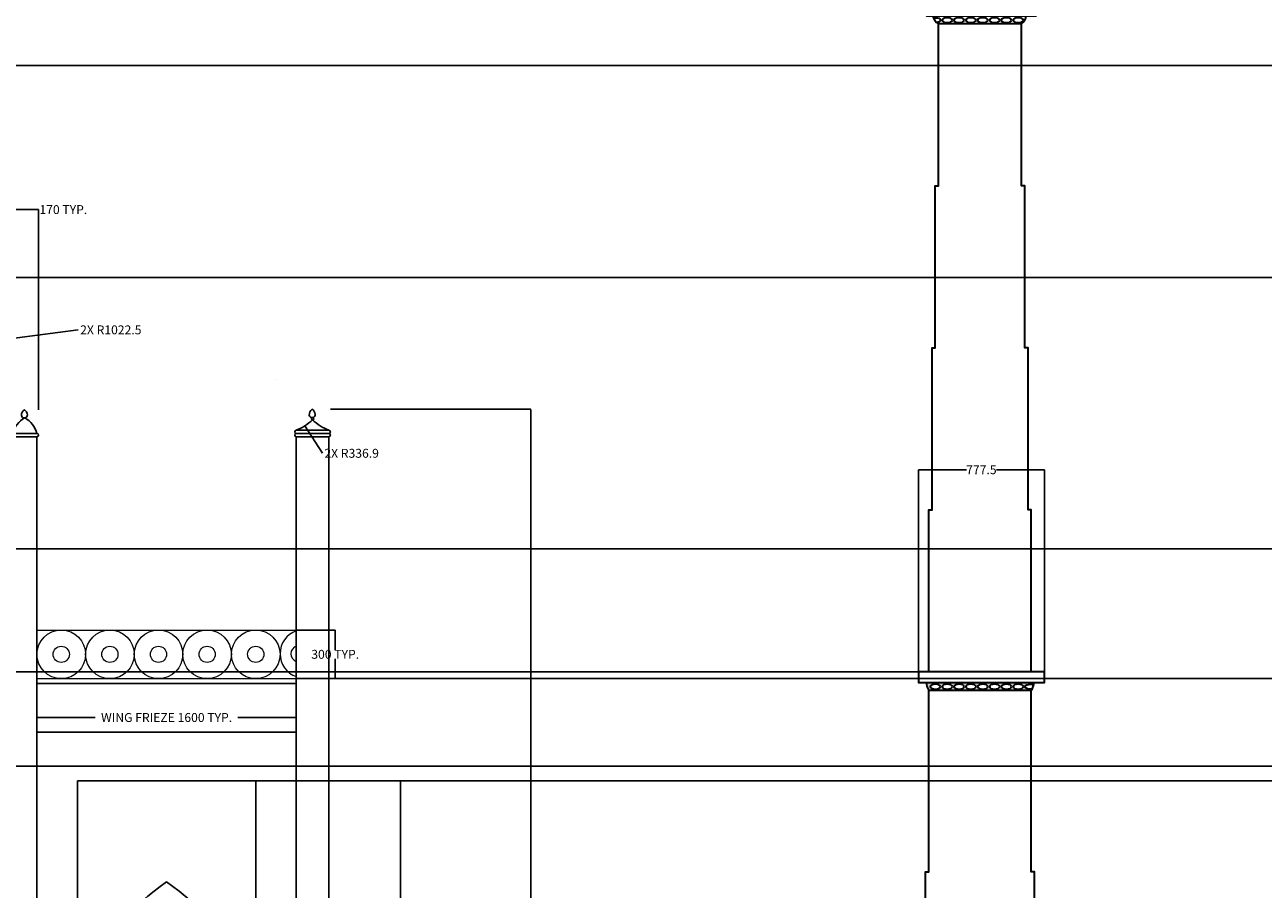
# Model space of a CAD drawing. Units: millimetres. Extents: x 8570 to 49085, y 3782 to 24863.
# Tile 9 of 15: x 27529 to 35169, y 12499 to 17835. Entities that reach past the tile are written whole.
import ezdxf

# ---------------------------------------------------------------- set-up
doc = ezdxf.new("R2010")
doc.units = ezdxf.units.MM
doc.header["$MEASUREMENT"] = 0
doc.header["$PDMODE"] = 3
for name, color, linetype, lineweight in [('A-ANNO-DIMS', 2, 'Continuous', 18), ('A-ELEV', 7, 'Continuous', 25), ('A-ELEV-ARCH', 7, 'Continuous', 25), ('A-ELEV-MNRT', 7, 'Continuous', 30), ('A-ELEV-ORNM', 7, 'Continuous', 13), ('A-ELEV-PIER', 7, 'Continuous', 25)]:
    doc.layers.add(name, color=color, linetype=linetype, lineweight=lineweight)
doc.styles.get("Standard").update_dxf_attribs({"font": 'arial.ttf'})
doc.dimstyles.get("Standard").update_dxf_attribs({"dimtxt": 55, "dimasz": 0.18, "dimexe": 0.18, "dimexo": 0.0625, "dimgap": 0.09, "dimtad": 0, "dimtih": 1, "dimtoh": 1, "dimdec": 0, "dimzin": 0, "dimdsep": 46, "dimtxsty": 'Standard', "dimcen": 0.09, "dimadec": 0, "dimazin": 0, "dimtfac": 1, "dimtdec": 0, "dimtofl": 0, "dimtmove": 0, "dimatfit": 3, "dimfxl": 1, "dimtolj": 1, "dimtzin": 0, "dimarcsym": 0})

# ---------------------------------------------------------------- blocks, each defined once
blk = doc.blocks.new('MINARET-ELEV')
h = blk.add_hatch(color=256)
h.dxf.hatch_style = 1
edge = h.paths.add_edge_path()
edge.add_arc((788.1, 7879), 96, 347.52389, 357.31225, ccw=False)
edge.add_ellipse((859.2, 7847.7), major_axis=(31.8, 0), ratio=0.472441, start_angle=385.01443, end_angle=315.51296)
edge.add_arc((788.1, 7879), 96, 325.26025, 332.17741, ccw=False)
edge.add_line((867, 7824.3), (235, 7824.3))
edge.add_arc((313.9, 7879), 96, 182.68775, 214.73975, ccw=False)
edge.add_line((218, 7874.5), (884, 7874.5))
edge = h.paths.add_edge_path(flags=16)
edge.add_ellipse((494.2, 7847.7), major_axis=(31.8, 0), ratio=0.472441, start_angle=0, end_angle=360, ccw=False)
edge = h.paths.add_edge_path(flags=16)
edge.add_ellipse((567.2, 7847.7), major_axis=(31.8, 0), ratio=0.472441, start_angle=0, end_angle=360, ccw=False)
edge = h.paths.add_edge_path(flags=16)
edge.add_ellipse((421.2, 7847.7), major_axis=(31.8, 0), ratio=0.472441, start_angle=0, end_angle=360, ccw=False)
edge = h.paths.add_edge_path(flags=16)
edge.add_ellipse((640.2, 7847.7), major_axis=(31.8, 0), ratio=0.472441, start_angle=0, end_angle=360, ccw=False)
edge = h.paths.add_edge_path(flags=16)
edge.add_ellipse((348.2, 7847.7), major_axis=(31.8, 0), ratio=0.472441, start_angle=0, end_angle=360, ccw=False)
edge = h.paths.add_edge_path(flags=16)
edge.add_ellipse((713.2, 7847.7), major_axis=(31.8, 0), ratio=0.472441, start_angle=0, end_angle=360, ccw=False)
edge = h.paths.add_edge_path(flags=16)
edge.add_ellipse((275.2, 7847.7), major_axis=(31.8, 0), ratio=0.472441, start_angle=0, end_angle=360, ccw=False)
edge = h.paths.add_edge_path(flags=16)
edge.add_ellipse((786.2, 7847.7), major_axis=(31.8, 0), ratio=0.472441, start_angle=0, end_angle=360, ccw=False)
h = blk.add_hatch(color=256)
h.dxf.hatch_style = 1
edge = h.paths.add_edge_path()
edge.add_arc((940, 4615.3), 25, 270, 450, ccw=False)
edge.add_line((940, 4590.3), (160, 4590.3))
edge.add_arc((160, 4615.3), 25, 217.6761, 270, ccw=False)
edge.add_ellipse((127.2, 4613.7), major_axis=(31.8, 0), ratio=0.472441, start_angle=313.43175, end_angle=411.74889)
edge.add_arc((160, 4615.3), 25, 450, 510.08055, ccw=False)
edge.add_line((160, 4640.3), (940, 4640.3))
edge = h.paths.add_edge_path(flags=16)
edge.add_ellipse((347.2, 4613.7), major_axis=(31.8, 0), ratio=0.472441, start_angle=0, end_angle=360, ccw=False)
edge = h.paths.add_edge_path(flags=16)
edge.add_ellipse((420.2, 4613.7), major_axis=(31.8, 0), ratio=0.472441, start_angle=0, end_angle=360, ccw=False)
edge = h.paths.add_edge_path(flags=16)
edge.add_ellipse((274.2, 4613.7), major_axis=(31.8, 0), ratio=0.472441, start_angle=0, end_angle=360, ccw=False)
edge = h.paths.add_edge_path(flags=16)
edge.add_ellipse((493.2, 4613.7), major_axis=(31.8, 0), ratio=0.472441, start_angle=0, end_angle=360, ccw=False)
edge = h.paths.add_edge_path(flags=16)
edge.add_ellipse((198.8, 4613.7), major_axis=(31.8, 0), ratio=0.472441, start_angle=0, end_angle=360, ccw=False)
edge = h.paths.add_edge_path(flags=16)
edge.add_ellipse((566.2, 4613.7), major_axis=(31.8, 0), ratio=0.472441, start_angle=0, end_angle=360, ccw=False)
edge = h.paths.add_edge_path(flags=16)
edge.add_ellipse((639.2, 4613.7), major_axis=(31.8, 0), ratio=0.472441, start_angle=0, end_angle=360, ccw=False)
edge = h.paths.add_edge_path(flags=16)
edge.add_ellipse((712.2, 4613.7), major_axis=(31.8, 0), ratio=0.472441, start_angle=0, end_angle=360, ccw=False)
edge = h.paths.add_edge_path(flags=16)
edge.add_ellipse((785.2, 4613.7), major_axis=(31.8, 0), ratio=0.472441, start_angle=0, end_angle=360, ccw=False)
edge = h.paths.add_edge_path(flags=16)
edge.add_ellipse((858.2, 4613.7), major_axis=(31.8, 0), ratio=0.472441, start_angle=0, end_angle=360, ccw=False)
edge = h.paths.add_edge_path(flags=16)
edge.add_ellipse((931.2, 4613.7), major_axis=(31.8, 0), ratio=0.472441, start_angle=0, end_angle=360, ccw=False)
for p, q in [((851, 12922), (257.5, 12922)), ((257.5, 12922), (257.5, 12872)), ((851, 12922), (851, 12872)), ((851, 12897), (257.5, 12897)), ((851, 12872), (257.5, 12872)), ((298, 12162), (298, 12872)), ((556.7, 12843), (552, 12843)), ((815.5, 12162), (815.5, 12872)), ((348, 12162), (348, 12766.4)), ((423, 12162), (423, 12760.1)), ((765.5, 12162), (765.5, 12770.9)), ((690.5, 12162), (690.5, 12757.3)), ((815.5, 12162), (298, 12162)), ((807, 11939), (295, 11939)), ((867, 7824.3), (235, 7824.3)), ((867, 7824.3), (235, 7824.3)), ((160, 4590.3), (940, 4590.3)), ((165, 4590.3), (935, 4590.3)), ((905, 4590.3), (195, 4590.3)), ((300, 0), (300, 1321)), ((800, 0), (800, 1321)), ((1100, 0), (1100, 1321))]:
    blk.add_line(p, q)
blk.add_lwpolyline([(512, 13519.5, -0.216309), (551.3, 13585.8, -0.244698), (591, 13509.3, -0.244698)], format="xyb")
for points in [[(554, 13300, -0.140093), (458.9, 13405.9, -0.184272)], [(554, 13300, 0.140093), (646.7, 13408, 0.184272)]]:
    blk.add_lwpolyline(points, format="xyb", close=True)
for points in [[(815.5, 12072.5), (298, 12072.5), (298, 12162), (815.5, 12162)], [(898, 12072.5), (220.5, 12072.5), (220.5, 11989.2), (898, 11989.2)], [(948, 7939), (170.5, 7939), (170.5, 7874.5), (948, 7874.5)], [(997, 4705), (119.5, 4705), (119.5, 4640.5), (997, 4640.5)]]:
    blk.add_lwpolyline(points, close=True)
for points in [[(235, 7939), (235, 8939), (255, 8939), (255, 9939), (275, 9939), (275, 10939), (295, 10939), (295, 11939)], [(867, 7939), (867, 8939), (847, 8939), (847, 9939), (827, 9939), (827, 10939), (807, 10939), (807, 11939)], [(195, 4705), (195, 5705), (215, 5705), (215, 6705), (235, 6705), (235, 7824.3)], [(907, 4705), (907, 5705), (887, 5705), (887, 6705), (867, 6705), (867, 7824.3)], [(135, 1321), (135, 2321), (155, 2321), (155, 3321), (175, 3321), (175, 4321), (195, 4321), (195, 4590.3)], [(965, 1321), (965, 2321), (945, 2321), (945, 3321), (925, 3321), (925, 4321), (905, 4321), (905, 4590.3)], [(0, 1321), (1100, 1321)], [(0, 1246), (1100, 1246)]]:
    blk.add_lwpolyline(points)
for centre, radius in [((552, 13415.4), 63.1), ((554, 13261.5), 38.5)]:
    blk.add_circle(centre, radius)
for centre, radius, start, end in [((552, 13518.5), 40.1, 178.61203, 346.69346), ((554, 12961.3), 261.7, 351.36698, 188.63302), ((330.8, 12000.6), 71.3, 189.21146, 239.80255), ((759.2, 12000.8), 78.1, 307.68318, 351.42034), ((313.9, 7879), 96, 182.68775, 214.73975), ((788.1, 7879), 96, 325.26025, 357.31225), ((160, 4615.3), 25, 90, 270), ((940, 4615.3), 25, 270, 90)]:
    blk.add_arc(centre, radius, start, end)
at = {"extrusion": (0, 0, -1)}
for centre, start_param, end_param in [((275.2, 11962.4), -1.939365, 1.327018), ((348.2, 11962.4), -6.283185, 0), ((421.2, 11962.4), -6.283185, 0), ((494.2, 11962.4), -6.283185, 0), ((567.2, 11962.4), -6.283185, 0), ((640.2, 11962.4), -6.283185, 0), ((713.2, 11962.4), -6.283185, 0), ((786.2, 11962.4), -6.283185, 0), ((275.2, 7847.7), -6.283185, 0), ((348.2, 7847.7), -6.283185, 0), ((421.2, 7847.7), -6.283185, 0), ((494.2, 7847.7), -6.283185, 0), ((567.2, 7847.7), -6.283185, 0), ((640.2, 7847.7), -6.283185, 0), ((713.2, 7847.7), -6.283185, 0), ((786.2, 7847.7), -6.283185, 0), ((859.2, 7847.7), -5.160703, -0.779193), ((127.2, 4613.7), -1.214257, 1.150222), ((198.8, 4613.7), -6.283185, 0), ((274.2, 4613.7), -6.283185, 0), ((347.2, 4613.7), -6.283185, 0), ((420.2, 4613.7), -6.283185, 0), ((493.2, 4613.7), -6.283185, 0), ((566.2, 4613.7), -6.283185, 0), ((639.2, 4613.7), -6.283185, 0), ((712.2, 4613.7), -6.283185, 0), ((785.2, 4613.7), -6.283185, 0), ((858.2, 4613.7), -6.283185, 0), ((931.2, 4613.7), -6.283185, 0)]:
    blk.add_ellipse(centre, major_axis=(31.8, 0), ratio=0.472441, start_param=start_param, end_param=end_param, dxfattribs=at)
for points in [[(554.4, 12843), (553.6, 12843), (500.8, 12843), (391.9, 12680.1), (321.9, 12795.7), (298, 12872)], [(554.4, 12843), (555.2, 12843), (607.9, 12843), (716.8, 12680.1), (786.9, 12795.7), (815.5, 12872)]]:
    blk.add_open_spline(points, degree=3, knots=[136.061972, 136.061972, 136.061972, 136.061972, 139.000899, 330.944902, 463.724089, 463.724089, 463.724089, 463.724089])
blk = doc.blocks.new('PAVILION-EDGE-PINNACLE')
for p, q in [((10, 8089.5), (160, 8089.5)), ((10, 0), (10, 8069.5)), ((10, 8069.5), (160, 8069.5)), ((160, 0), (160, 8069.5)), ((160, 0), (160, 6876.5)), ((10, 0), (10, 6246.5))]:
    blk.add_line(p, q)
blk.add_lwpolyline([(101.6, 8204.8, 0.216309), (82.9, 8236.3, 0.244698), (64, 8200, 0.244698)], format="xyb")
for centre, radius, start, end in [((153, 8055.1), 147, 117.52778, 166.47476), ((82.6, 8204.4), 19, 193.30654, 1.38797), ((17, 8055.1), 147, 13.52524, 62.47222), ((10, 8079.5), 10, 90, 270), ((160, 8079.5), 10, 270, 90)]:
    blk.add_arc(centre, radius, start, end)
blk = doc.blocks.new('WING-END-PINNACLE')
for p, q in [((10, 8109.5), (210, 8109.5)), ((10, 8089.5), (210, 8089.5)), ((10, 0), (10, 8069.5)), ((10, 8069.5), (210, 8069.5)), ((210, 0), (210, 8069.5))]:
    blk.add_line(p, q)
blk.add_lwpolyline([(127.1, 8207.4, 0.216309), (108.4, 8238.9, 0.244698), (89.5, 8202.5, 0.244698)], format="xyb")
blk.add_circle((110.5, 8181), 7.02)
for centre, radius, start, end in [((108.1, 8206.9), 19, 193.30654, 1.38797), ((10, 8099.5), 10, 90, 270), ((-119.7, 8420.4), 336.9, 292.6494, 312.99463), ((340.2, 8421.1), 337.7, 227.0303, 247.32566), ((210, 8099.5), 10, 270, 90), ((10, 8079.5), 10, 90, 270), ((210, 8079.5), 10, 270, 90)]:
    blk.add_arc(centre, radius, start, end)
blk = doc.blocks.new('WING-RING-FRIEZE')
for p, q in [((0, 300), (1600, 300)), ((0, 0), (1600, 0))]:
    blk.add_line(p, q)
for centre, radius in [((150, 150), 150), ((450, 150), 150), ((750, 150), 150), ((1050, 150), 150), ((1349.9, 150), 150), ((150, 150), 50), ((450, 150), 50), ((750, 150), 50), ((1050, 150), 50), ((1349.9, 150), 50)]:
    blk.add_circle(centre, radius)
for centre, radius in [((1649.9, 153.7), 150), ((1616.6, 153.7), 50)]:
    blk.add_arc(centre, radius, 109.41717, 250.58283)
blk = doc.blocks.new('WING-TALL-ARCH')
for p, q in [((0, 5946.5), (1100, 5946.5)), ((0, 0), (0, 5946.5)), ((1100, 0), (1100, 5946.5)), ((0, 3123.2), (1100, 3123.2))]:
    blk.add_line(p, q)
for points in [[(47.9, 4748, -0.124525), (550, 5321.3, -0.124525)], [(1052.1, 4748, 0.124525), (550, 5321.3, 0.124525)]]:
    blk.add_lwpolyline(points, format="xyb")
for centre, start, end in [((817.4, 4459.8), 159.46554, 174.14569), ((282.6, 4459.8), 5.85431, 20.53446)]:
    blk.add_arc(centre, 821.7, start, end)
blk = doc.blocks.new('*D15')
at = {"layer": 'A-ANNO-DIMS', "color": 0, "lineweight": -2, "transparency": 16777216}
for p, q in [((33971.1, 19487.3), (36009.1, 19487.3)), ((36008.9, 19487.1), (36008.9, 12722.6)), ((36008.9, 5901.7), (36008.9, 12666.2)), ((33971.1, 5901.5), (36009.1, 5901.5))]:
    blk.add_line(p, q, dxfattribs=at)
at = {"layer": 'A-ANNO-DIMS', "color": 0, "transparency": 16777216}
for points in [[(36008.8, 19487.1), (36008.9, 19487.1), (36008.9, 19487.3)], [(36008.8, 5901.7), (36008.9, 5901.7), (36008.9, 5901.5)]]:
    blk.add_solid(points, dxfattribs=at)
at = {"layer": 'Defpoints', "color": 0, "transparency": 16777216}
for p in [(33971, 19487.3), (36008.9, 19487.3), (33971, 5901.5)]:
    blk.add_point(p, dxfattribs=at)
at = {"layer": 'A-ANNO-DIMS', "color": 0, "transparency": 16777216, "insert": (36008.9, 12694.4), "char_height": 55, "attachment_point": 5}
blk.add_mtext('\\A1;MINARET 13586 TYP.', dxfattribs=at)
blk = doc.blocks.new('*D22')
at = {"layer": 'A-ANNO-DIMS', "color": 0, "lineweight": -2, "transparency": 16777216}
for p, q in [((27444, 15458.9), (27444, 16694.5)), ((27444.2, 16694.3), (27613.8, 16694.3)), ((27614, 15458.9), (27614, 16694.5)), ((27614, 16694.3), (27614.2, 16694.3))]:
    blk.add_line(p, q, dxfattribs=at)
at = {"layer": 'A-ANNO-DIMS', "color": 0, "transparency": 16777216}
for points in [[(27444.2, 16694.3), (27444.2, 16694.3), (27444, 16694.3)], [(27613.8, 16694.3), (27613.8, 16694.3), (27614, 16694.3)]]:
    blk.add_solid(points, dxfattribs=at)
at = {"layer": 'Defpoints', "color": 0, "transparency": 16777216}
for p in [(27614, 16694.3), (27444, 15458.8), (27614, 15458.8)]:
    blk.add_point(p, dxfattribs=at)
at = {"layer": 'A-ANNO-DIMS', "color": 0, "transparency": 16777216, "insert": (27766.9, 16694.3), "char_height": 55, "attachment_point": 5}
blk.add_mtext('\\A1;170 TYP.', dxfattribs=at)
blk = doc.blocks.new('*D23')
at = {"layer": 'A-ANNO-DIMS', "color": 0, "lineweight": -2, "transparency": 16777216}
for p, q in [((29414.1, 15461.4), (30650, 15461.4)), ((30649.8, 15461.2), (30649.8, 11370.5)), ((30649.8, 7222.7), (30649.8, 11313.4)), ((29414.1, 7222.5), (30650, 7222.5))]:
    blk.add_line(p, q, dxfattribs=at)
at = {"layer": 'A-ANNO-DIMS', "color": 0, "transparency": 16777216}
for points in [[(30649.8, 15461.2), (30649.9, 15461.2), (30649.8, 15461.4)], [(30649.8, 7222.7), (30649.9, 7222.7), (30649.8, 7222.5)]]:
    blk.add_solid(points, dxfattribs=at)
at = {"layer": 'Defpoints', "color": 0, "transparency": 16777216}
for p in [(29414, 15461.4), (30649.8, 15461.4), (29414, 7222.5)]:
    blk.add_point(p, dxfattribs=at)
at = {"layer": 'A-ANNO-DIMS', "color": 0, "transparency": 16777216, "insert": (30649.8, 11341.9), "char_height": 55, "attachment_point": 5}
blk.add_mtext('\\A1;WING PINNACLE 8239 TYP.', dxfattribs=at)
blk = doc.blocks.new('*D31')
at = {"layer": 'A-ANNO-DIMS', "color": 0, "lineweight": -2, "transparency": 16777216}
for p, q in [((28954.1, 13169), (29846.2, 13169)), ((29846, 13168.8), (29846, 10224.3)), ((29846, 7222.7), (29846, 10167.2)), ((28954.1, 7222.5), (29846.2, 7222.5))]:
    blk.add_line(p, q, dxfattribs=at)
at = {"layer": 'A-ANNO-DIMS', "color": 0, "transparency": 16777216}
for points in [[(29845.9, 13168.8), (29846, 13168.8), (29846, 13169)], [(29845.9, 7222.7), (29846, 7222.7), (29846, 7222.5)]]:
    blk.add_solid(points, dxfattribs=at)
at = {"layer": 'Defpoints', "color": 0, "transparency": 16777216}
for p in [(28954, 13169), (29846, 13169), (28954, 7222.5)]:
    blk.add_point(p, dxfattribs=at)
at = {"layer": 'A-ANNO-DIMS', "color": 0, "transparency": 16777216, "insert": (29846, 10195.7), "char_height": 55, "attachment_point": 5}
blk.add_mtext('\\A1;TALL ARCH 5947 TYP.', dxfattribs=at)
blk = doc.blocks.new('*D35')
at = {"layer": 'A-ANNO-DIMS', "color": 0, "lineweight": -2, "transparency": 16777216}
for p, q in [((27604, 13798.9), (27604, 13558.8)), ((29204, 13798.9), (29204, 13558.8)), ((27604.2, 13559), (27963.7, 13559)), ((29203.8, 13559), (28844.3, 13559))]:
    blk.add_line(p, q, dxfattribs=at)
at = {"layer": 'A-ANNO-DIMS', "color": 0, "transparency": 16777216}
for points in [[(27604.2, 13559), (27604.2, 13559), (27604, 13559)], [(29203.8, 13559), (29203.8, 13559), (29204, 13559)]]:
    blk.add_solid(points, dxfattribs=at)
at = {"layer": 'Defpoints', "color": 0, "transparency": 16777216}
for p in [(27604, 13799), (29204, 13799), (29204, 13559)]:
    blk.add_point(p, dxfattribs=at)
at = {"layer": 'A-ANNO-DIMS', "color": 0, "transparency": 16777216, "insert": (28404, 13559), "char_height": 55, "attachment_point": 5}
blk.add_mtext('\\A1;WING FRIEZE 1600 TYP.', dxfattribs=at)
blk = doc.blocks.new('*D36')
at = {"layer": 'A-ANNO-DIMS', "color": 0, "lineweight": -2, "transparency": 16777216}
for p, q in [((29204.1, 14099), (29444.2, 14099)), ((29444, 14098.8), (29444, 13977.2)), ((29444, 13799.2), (29444, 13920.8)), ((29204.1, 13799), (29444.2, 13799))]:
    blk.add_line(p, q, dxfattribs=at)
at = {"layer": 'A-ANNO-DIMS', "color": 0, "transparency": 16777216}
for points in [[(29444, 14098.8), (29444, 14098.8), (29444, 14099)], [(29444, 13799.2), (29444, 13799.2), (29444, 13799)]]:
    blk.add_solid(points, dxfattribs=at)
at = {"layer": 'Defpoints', "color": 0, "transparency": 16777216}
for p in [(29204, 14099), (29444, 14099), (29204, 13799)]:
    blk.add_point(p, dxfattribs=at)
at = {"layer": 'A-ANNO-DIMS', "color": 0, "transparency": 16777216, "insert": (29444, 13949), "char_height": 55, "attachment_point": 5}
blk.add_mtext('\\A1;300 TYP.', dxfattribs=at)
blk = doc.blocks.new('*D50')
at = {"layer": 'A-ANNO-DIMS', "color": 0, "lineweight": -2, "transparency": 16777216}
for p, q in [((22407.6, 13259), (36055.2, 13259)), ((36055, 13258.8), (36055, 12570.2)), ((36055, 11825.2), (36055, 12513.8)), ((24254.1, 11825), (36055.2, 11825))]:
    blk.add_line(p, q, dxfattribs=at)
at = {"layer": 'A-ANNO-DIMS', "color": 0, "transparency": 16777216}
for points in [[(36055, 13258.8), (36055, 13258.8), (36055, 13259)], [(36055, 11825.2), (36055, 11825.2), (36055, 11825)]]:
    blk.add_solid(points, dxfattribs=at)
at = {"layer": 'Defpoints', "color": 0, "transparency": 16777216}
for p in [(22407.5, 13259), (36055, 13259), (24254, 11825)]:
    blk.add_point(p, dxfattribs=at)
at = {"layer": 'A-ANNO-DIMS', "color": 0, "transparency": 16777216, "insert": (36055, 12542), "char_height": 55, "attachment_point": 5}
blk.add_mtext('\\A1;1434', dxfattribs=at)
blk = doc.blocks.new('*D51')
at = {"layer": 'A-ANNO-DIMS', "color": 0, "lineweight": -2, "transparency": 16777216}
for p, q in [((25004.1, 14600), (36055.2, 14600)), ((36055, 14599.8), (36055, 13957.7)), ((36055, 13259.2), (36055, 13901.3)), ((22407.6, 13259), (36055.2, 13259))]:
    blk.add_line(p, q, dxfattribs=at)
at = {"layer": 'A-ANNO-DIMS', "color": 0, "transparency": 16777216}
for points in [[(36055, 14599.8), (36055, 14599.8), (36055, 14600)], [(36055, 13259.2), (36055, 13259.2), (36055, 13259)]]:
    blk.add_solid(points, dxfattribs=at)
at = {"layer": 'Defpoints', "color": 0, "transparency": 16777216}
for p in [(25004, 14600), (36055, 14600), (22407.5, 13259)]:
    blk.add_point(p, dxfattribs=at)
at = {"layer": 'A-ANNO-DIMS', "color": 0, "transparency": 16777216, "insert": (36055, 13929.5), "char_height": 55, "attachment_point": 5}
blk.add_mtext('\\A1;1341', dxfattribs=at)
blk = doc.blocks.new('*D53')
at = {"layer": 'A-ANNO-DIMS', "color": 0, "lineweight": -2, "transparency": 16777216}
for p, q in [((26017.6, 17582.8), (36055.2, 17582.8)), ((36055, 17582.6), (36055, 16957.5)), ((36055, 16276), (36055, 16901.1)), ((25347.4, 16275.8), (36055.2, 16275.8))]:
    blk.add_line(p, q, dxfattribs=at)
at = {"layer": 'A-ANNO-DIMS', "color": 0, "transparency": 16777216}
for points in [[(36055, 17582.6), (36055, 17582.6), (36055, 17582.8)], [(36055, 16276), (36055, 16276), (36055, 16275.8)]]:
    blk.add_solid(points, dxfattribs=at)
at = {"layer": 'Defpoints', "color": 0, "transparency": 16777216}
for p in [(26017.6, 17582.8), (36055, 17582.8), (25347.3, 16275.8)]:
    blk.add_point(p, dxfattribs=at)
at = {"layer": 'A-ANNO-DIMS', "color": 0, "transparency": 16777216, "insert": (36055, 16929.3), "char_height": 55, "attachment_point": 5}
blk.add_mtext('\\A1;1307', dxfattribs=at)
blk = doc.blocks.new('*D54')
at = {"layer": 'A-ANNO-DIMS', "color": 0, "lineweight": -2, "transparency": 16777216}
for p, q in [((24765.7, 21387.4), (36055.2, 21387.4)), ((36055, 21387.2), (36055, 19513.3)), ((36055, 17583), (36055, 19456.9)), ((26017.6, 17582.8), (36055.2, 17582.8))]:
    blk.add_line(p, q, dxfattribs=at)
at = {"layer": 'A-ANNO-DIMS', "color": 0, "transparency": 16777216}
for points in [[(36055, 21387.2), (36055, 21387.2), (36055, 21387.4)], [(36055, 17583), (36055, 17583), (36055, 17582.8)]]:
    blk.add_solid(points, dxfattribs=at)
at = {"layer": 'Defpoints', "color": 0, "transparency": 16777216}
for p in [(24765.6, 21387.4), (36055, 21387.4), (26017.6, 17582.8)]:
    blk.add_point(p, dxfattribs=at)
at = {"layer": 'A-ANNO-DIMS', "color": 0, "transparency": 16777216, "insert": (36055, 19485.1), "char_height": 55, "attachment_point": 5}
blk.add_mtext('\\A1;3804.6', dxfattribs=at)
blk = doc.blocks.new('*D60')
at = {"layer": 'A-ANNO-DIMS', "color": 0, "lineweight": -2, "transparency": 16777216}
for p, q in [((33041.4, 13840.5), (8684.3, 13840.5)), ((8684.5, 13840.3), (8684.5, 12251.7)), ((8684.5, 10606.7), (8684.5, 12195.3)), ((32990.4, 10606.5), (8684.3, 10606.5))]:
    blk.add_line(p, q, dxfattribs=at)
at = {"layer": 'A-ANNO-DIMS', "color": 0, "transparency": 16777216}
for points in [[(8684.5, 13840.3), (8684.5, 13840.3), (8684.5, 13840.5)], [(8684.5, 10606.7), (8684.5, 10606.7), (8684.5, 10606.5)]]:
    blk.add_solid(points, dxfattribs=at)
at = {"layer": 'Defpoints', "color": 0, "transparency": 16777216}
for p in [(8684.5, 13840.5), (33041.5, 13840.5), (32990.5, 10606.5)]:
    blk.add_point(p, dxfattribs=at)
at = {"layer": 'A-ANNO-DIMS', "color": 0, "transparency": 16777216, "insert": (8684.5, 12223.5), "char_height": 55, "attachment_point": 5}
blk.add_mtext('\\A1;3234', dxfattribs=at)
blk = doc.blocks.new('*D61')
at = {"layer": 'A-ANNO-DIMS', "color": 0, "lineweight": -2, "transparency": 16777216}
for p, q in [((33091.4, 17974), (8684.3, 17974)), ((8684.5, 17973.8), (8684.5, 15935.4)), ((8684.5, 13840.7), (8684.5, 15879.1)), ((33041.4, 13840.5), (8684.3, 13840.5))]:
    blk.add_line(p, q, dxfattribs=at)
at = {"layer": 'A-ANNO-DIMS', "color": 0, "transparency": 16777216}
for points in [[(8684.5, 17973.8), (8684.5, 17973.8), (8684.5, 17974)], [(8684.5, 13840.7), (8684.5, 13840.7), (8684.5, 13840.5)]]:
    blk.add_solid(points, dxfattribs=at)
at = {"layer": 'Defpoints', "color": 0, "transparency": 16777216}
for p in [(8684.5, 17974), (33091.5, 17974), (33041.5, 13840.5)]:
    blk.add_point(p, dxfattribs=at)
at = {"layer": 'A-ANNO-DIMS', "color": 0, "transparency": 16777216, "insert": (8684.5, 15907.2), "char_height": 55, "attachment_point": 5}
blk.add_mtext('\\A1;4133.5', dxfattribs=at)
blk = doc.blocks.new('*D64')
at = {"layer": 'A-ANNO-DIMS', "color": 0, "lineweight": -2, "transparency": 16777216}
for p, q in [((33041.5, 13840.6), (33041.5, 15088.7)), ((33041.7, 15088.5), (33337.4, 15088.5)), ((33818.8, 15088.5), (33523.1, 15088.5)), ((33819, 13840.6), (33819, 15088.7))]:
    blk.add_line(p, q, dxfattribs=at)
at = {"layer": 'A-ANNO-DIMS', "color": 0, "transparency": 16777216}
for points in [[(33041.7, 15088.5), (33041.7, 15088.5), (33041.5, 15088.5)], [(33818.8, 15088.5), (33818.8, 15088.5), (33819, 15088.5)]]:
    blk.add_solid(points, dxfattribs=at)
at = {"layer": 'Defpoints', "color": 0, "transparency": 16777216}
for p in [(33819, 15088.5), (33041.5, 13840.5), (33819, 13840.5)]:
    blk.add_point(p, dxfattribs=at)
at = {"layer": 'A-ANNO-DIMS', "color": 0, "transparency": 16777216, "insert": (33430.2, 15088.5), "char_height": 55, "attachment_point": 5}
blk.add_mtext('\\A1;777.5', dxfattribs=at)
blk = doc.blocks.new('*D68')
at = {"layer": 'A-ANNO-DIMS', "color": 0, "lineweight": -2, "transparency": 16777216}
for p, q in [((29204.1, 13799), (36055.2, 13799)), ((36055, 13798.8), (36055, 13512.2)), ((36055, 13169.2), (36055, 13455.8)), ((28954.1, 13169), (36055.2, 13169))]:
    blk.add_line(p, q, dxfattribs=at)
at = {"layer": 'A-ANNO-DIMS', "color": 0, "transparency": 16777216}
for points in [[(36055, 13798.8), (36055, 13798.8), (36055, 13799)], [(36055, 13169.2), (36055, 13169.2), (36055, 13169)]]:
    blk.add_solid(points, dxfattribs=at)
at = {"layer": 'Defpoints', "color": 0, "transparency": 16777216}
for p in [(29204, 13799), (36055, 13799), (28954, 13169)]:
    blk.add_point(p, dxfattribs=at)
at = {"layer": 'A-ANNO-DIMS', "color": 0, "transparency": 16777216, "insert": (36055, 13484), "char_height": 55, "attachment_point": 5}
blk.add_mtext('\\A1;630', dxfattribs=at)
blk = doc.blocks.new('*D87')
at = {"layer": 'A-ANNO-DIMS', "color": 0, "lineweight": -2, "transparency": 16777216}
for p, q in [((27859.4, 15951.8), (27251.1, 15873.5)), ((26236.7, 15742.8), (26236.9, 15742.8)), ((26236.8, 15742.7), (26236.8, 15742.9))]:
    blk.add_line(p, q, dxfattribs=at)
at = {"layer": 'A-ANNO-DIMS', "color": 0, "transparency": 16777216}
blk.add_solid([(27251.1, 15873.5), (27251.1, 15873.4), (27251, 15873.4)], dxfattribs=at)
at = {"layer": 'Defpoints', "color": 0, "transparency": 16777216}
for p in [(27251, 15873.4), (26236.8, 15742.8)]:
    blk.add_point(p, dxfattribs=at)
at = {"layer": 'A-ANNO-DIMS', "color": 0, "transparency": 16777216, "insert": (28059.8, 15951.8), "char_height": 55, "attachment_point": 5}
blk.add_mtext('\\A1;2X R1022.5', dxfattribs=at)
blk = doc.blocks.new('*D93')
at = {"layer": 'A-ANNO-DIMS', "color": 0, "lineweight": -2, "transparency": 16777216}
for p, q in [((29074.2, 15642.9), (29074.4, 15642.9)), ((29074.3, 15642.8), (29074.3, 15643)), ((29366.4, 15189.9), (29257, 15359.6)), ((29366.6, 15189.9), (29366.4, 15189.9))]:
    blk.add_line(p, q, dxfattribs=at)
at = {"layer": 'A-ANNO-DIMS', "color": 0, "transparency": 16777216}
blk.add_solid([(29257, 15359.7), (29256.9, 15359.6), (29256.9, 15359.8)], dxfattribs=at)
at = {"layer": 'Defpoints', "color": 0, "transparency": 16777216}
for p in [(29074.3, 15642.9), (29256.9, 15359.8)]:
    blk.add_point(p, dxfattribs=at)
at = {"layer": 'A-ANNO-DIMS', "color": 0, "transparency": 16777216, "insert": (29545.4, 15189.9), "char_height": 55, "attachment_point": 5}
blk.add_mtext('\\A1;2X R336.9', dxfattribs=at)

msp = doc.modelspace()

# ---------------------------------------------------------------- linework, layer by layer
at = {"layer": 'A-ELEV'}
for p, q in [((27604, 13769), (29204, 13769)), ((27604, 13469), (29204, 13469))]:
    msp.add_line(p, q, dxfattribs=at)

# ---------------------------------------------------------------- block references
at = {"layer": 'A-ELEV-ARCH'}
msp.add_blockref('WING-TALL-ARCH', (27854, 7222.5), dxfattribs=at)
at = {"layer": 'A-ELEV-MNRT'}
msp.add_blockref('MINARET-ELEV', (32871, 5901.5), dxfattribs=at)
at = {"layer": 'A-ELEV-ORNM'}
msp.add_blockref('WING-RING-FRIEZE', (27604, 13799), dxfattribs=at)
at = {"layer": 'A-ELEV-PIER'}
for name, p in [('PAVILION-EDGE-PINNACLE', (27444, 7222.5)), ('WING-END-PINNACLE', (29194, 7222.5))]:
    msp.add_blockref(name, p, dxfattribs=at)

# ---------------------------------------------------------------- dimensions: what is measured, and where the dimension line sits
at = {"layer": 'A-ANNO-DIMS'}
for base, p1, p2, override, picture, middle in [((36055, 21387.41), (26017.56, 17582.82), (24765.63, 21387.41), {"dimdec": 1, "dimlfac": 1, "dimrnd": 0, "dimzin": 0, "dimdsep": 46, "dimlunit": 2}, '*D54', (36055, 19485.11)), ((8684.5, 17974), (33041.5, 13840.5), (33091.5, 17974), {"dimdec": 1, "dimlfac": 1, "dimrnd": 0, "dimzin": 0, "dimdsep": 46, "dimlunit": 2}, '*D61', (8684.5, 15907.25)), ((36055, 17582.82), (25347.34, 16275.82), (26017.56, 17582.82), {"dimdec": 0, "dimlfac": 1, "dimrnd": 0, "dimzin": 0, "dimdsep": 46, "dimlunit": 2}, '*D53', (36055, 16929.32)), ((36055, 14600), (22407.5, 13259), (25004, 14600), {"dimdec": 0, "dimlfac": 1, "dimrnd": 0, "dimzin": 0, "dimdsep": 46, "dimlunit": 2}, '*D51', (36055, 13929.5)), ((8684.5, 13840.5), (32990.5, 10606.5), (33041.5, 13840.5), {"dimdec": 0, "dimlfac": 1, "dimrnd": 0, "dimzin": 0, "dimdsep": 46, "dimlunit": 2}, '*D60', (8684.5, 12223.5)), ((36055, 13799), (28954, 13169), (29204, 13799), {"dimdec": 0, "dimlfac": 1, "dimrnd": 0, "dimzin": 0, "dimdsep": 46, "dimlunit": 2}, '*D68', (36055, 13484)), ((36055, 13259), (24254, 11825), (22407.5, 13259), {"dimdec": 0, "dimlfac": 1, "dimrnd": 0, "dimzin": 0, "dimdsep": 46, "dimlunit": 2}, '*D50', (36055, 12542))]:
    dim = msp.add_linear_dim(base=base, p1=p1, p2=p2, angle=90, dimstyle='Standard', override=override, dxfattribs=at)
    dim.commit()
    dim.dimension.update_dxf_attribs({"geometry": picture, "text_midpoint": middle})
for base, p1, p2, text, picture, middle in [((36008.87, 19487.32), (33971, 5901.5), (33971, 19487.32), 'MINARET <> TYP.', '*D15', (36008.87, 12694.41)), ((30649.83, 15461.36), (29414, 7222.5), (29414, 15461.36), 'WING PINNACLE <> TYP.', '*D23', (30649.83, 11341.93)), ((29444, 14099), (29204, 13799), (29204, 14099), '<> TYP.', '*D36', (29444, 13949)), ((29845.975, 13169), (28954, 7222.5), (28954, 13169), 'TALL ARCH <> TYP.', '*D31', (29845.975, 10195.75))]:
    dim = msp.add_linear_dim(base=base, p1=p1, p2=p2, angle=90, text=text, dimstyle='Standard', override={"dimdec": 0, "dimlfac": 1, "dimrnd": 0, "dimzin": 0, "dimdsep": 46, "dimlunit": 2}, dxfattribs=at)
    dim.commit()
    dim.dimension.update_dxf_attribs({"geometry": picture, "text_midpoint": middle})
for base, p1, p2, text, picture, middle in [((27614, 16694.3), (27444, 15458.84), (27614, 15458.84), '<> TYP.', '*D22', (27766.91, 16694.3)), ((29204, 13559), (27604, 13799), (29204, 13799), 'WING FRIEZE <> TYP.', '*D35', (28404, 13559))]:
    dim = msp.add_linear_dim(base=base, p1=p1, p2=p2, text=text, dimstyle='Standard', override={"dimdec": 0, "dimlfac": 1, "dimrnd": 0, "dimzin": 0, "dimdsep": 46, "dimlunit": 2}, dxfattribs=at)
    dim.commit()
    dim.dimension.update_dxf_attribs({"geometry": picture, "text_midpoint": middle})
for center, mpoint, picture, middle in [((26236.79, 15742.8), (27250.95, 15873.44), '*D87', (27859.45, 15951.82)), ((29074.27, 15642.9), (29256.87, 15359.8), '*D93', (29545.43, 15189.94))]:
    dim = msp.add_radius_dim(center=center, mpoint=mpoint, text='2X <>', dimstyle='Standard', override={"dimdec": 1, "dimlfac": 1, "dimrnd": 0, "dimzin": 0, "dimdsep": 46, "dimlunit": 2}, dxfattribs=at)
    dim.commit()
    dim.dimension.update_dxf_attribs({"geometry": picture, "text_midpoint": middle, "dimtype": 164})
dim = msp.add_linear_dim(base=(33819, 15088.5), p1=(33041.5, 13840.5), p2=(33819, 13840.5), dimstyle='Standard', override={"dimdec": 1, "dimlfac": 1, "dimrnd": 0, "dimzin": 0, "dimdsep": 46, "dimlunit": 2}, dxfattribs=at)
dim.commit()
dim.dimension.update_dxf_attribs({"geometry": '*D64', "text_midpoint": (33430.25, 15088.5)})

doc.saveas('drawing.dxf')
